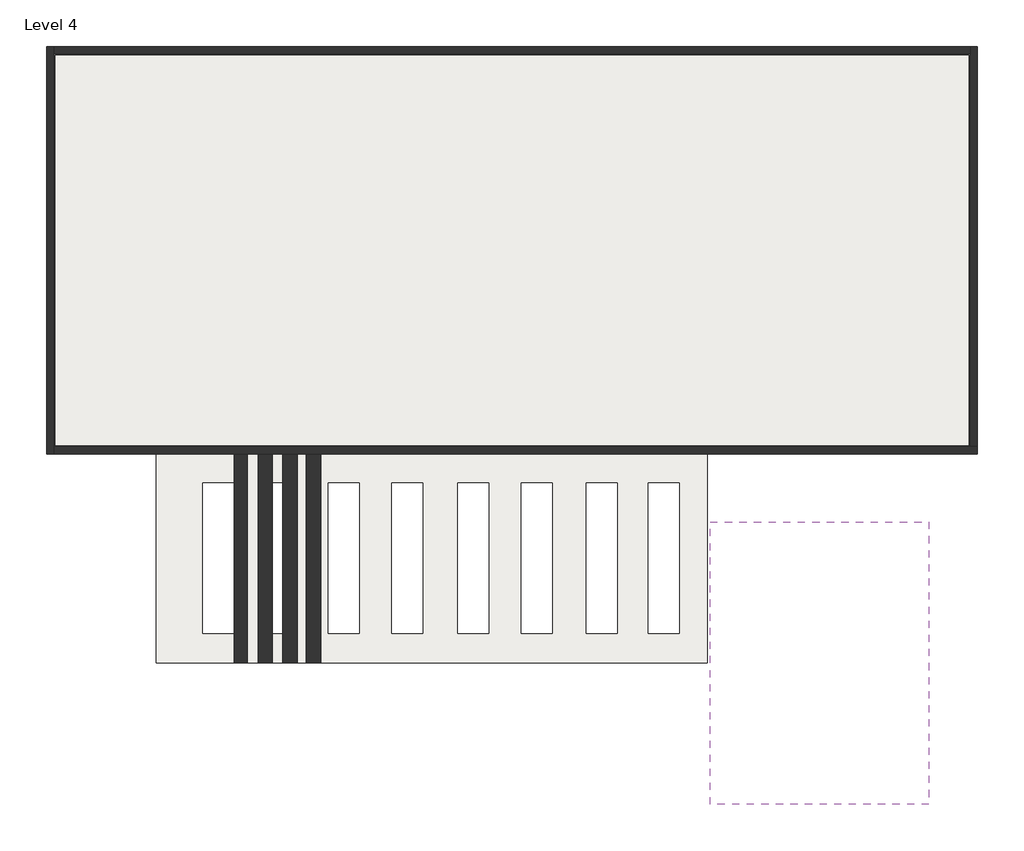
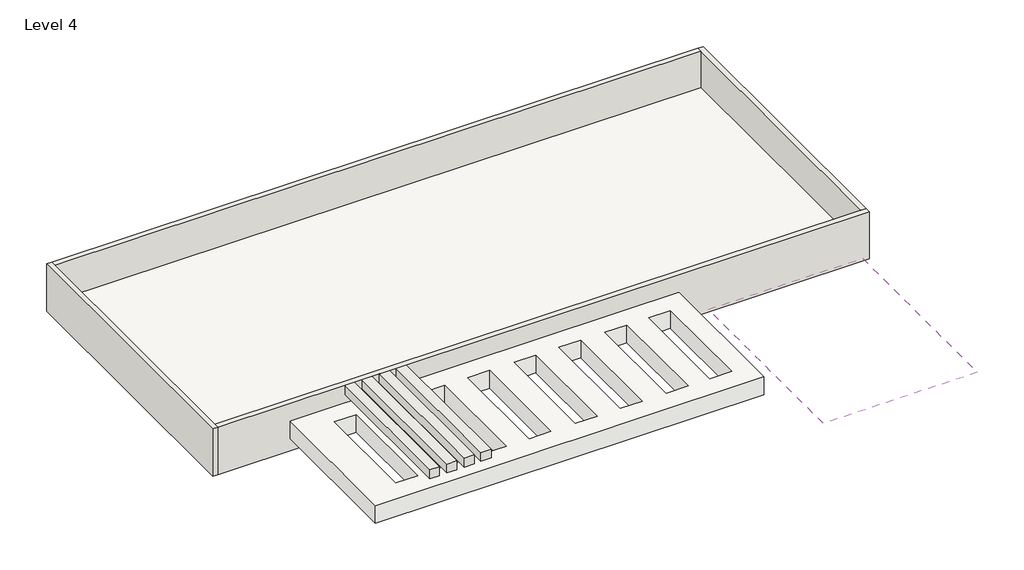
# One storey, incomplete: 5 walls, 3 roofs.
"""IFC4 building model written with IfcOpenShell, lengths in millimetres."""

from ifc_helpers import new_model, si_unit, frame, origin, place, context, project, spatial, polyline, outline, extrude, faceted_brep, transform, mapped, element, save
from components import walls_7_walls_7_6bd86e60

model = new_model("IFC4")

# Units and contexts
model_context = context("Model", 3, world=origin())
ifc_project = project(units=[si_unit("LENGTHUNIT", "METRE", prefix="MILLI")], contexts=[model_context])

# Site, building, storey
site = spatial("IfcSite", under=ifc_project)
building = spatial("IfcBuilding", under=site)
storey = spatial("IfcBuildingStorey", under=building, Name="Level 4", Elevation=10972.8)

# Roofs
placement = place(None, origin())
element("IfcRoof", 1, ObjectType="Generic - 12\"", at=placement, inside=storey, context=model_context, shape_type="SweptSolid", body=[
    extrude(outline(polyline([(-11592.9602581, 8068.7114178), (4110.5897419, 8068.7114178), (4110.5897419, 1363.1114178), (-11592.9602581, 1363.1114178), (-11592.9602581, 8068.7114178)])), frame((0.0, 0.0, 10972.8), z_axis=(0.0, 0.0, 1.0), x_axis=(1.0, 0.0, 0.0)), (0.0, 0.0, 1.0), 304.8),
])
element("IfcRoof", 2, ObjectType="Generic - 12\"", at=placement, inside=storey, context=model_context, shape_type="SweptSolid", body=[
    extrude(outline(polyline([(-337.4620963, 42.3114178), (3421.7379037, 42.3114178), (3421.7379037, -4809.0885822), (-337.4620963, -4809.0885822), (-337.4620963, 42.3114178)])), frame((0.0, 0.0, 11988.8), z_axis=(0.0, 0.0, 1.0), x_axis=(1.0, 0.0, 0.0)), (0.0, 0.0, 1.0), 304.8),
])
element("IfcRoof", 3, ObjectType="Generic - 18\"", at=placement, inside=storey, context=model_context, shape_type="SweptSolid", body=[
    extrude(outline(polyline([(-9855.5936547, 1337.7114178), (-388.2620963, 1337.7114178), (-388.2620963, -2383.3885822), (-9855.5936547, -2383.3885822), (-9855.5936547, 1337.7114178)]), holes=[polyline([(-8530.7557758, -1873.0263421), (-8530.7557758, 717.7736579), (-9064.1557758, 717.7736579), (-9064.1557758, -1873.0263421), (-8530.7557758, -1873.0263421)]), polyline([(-7438.5557758, -1873.0263421), (-7438.5557758, 717.7736579), (-7971.9557758, 717.7736579), (-7971.9557758, -1873.0263421), (-7438.5557758, -1873.0263421)]), polyline([(-6371.7557758, -1873.0263421), (-6371.7557758, 717.7736579), (-6905.1557758, 717.7736579), (-6905.1557758, -1873.0263421), (-6371.7557758, -1873.0263421)]), polyline([(-5279.5557758, -1873.0263421), (-5279.5557758, 717.7736579), (-5812.9557758, 717.7736579), (-5812.9557758, -1873.0263421), (-5279.5557758, -1873.0263421)]), polyline([(-4147.4620963, -1873.0263421), (-4147.4620963, 717.7736579), (-4680.8620963, 717.7736579), (-4680.8620963, -1873.0263421), (-4147.4620963, -1873.0263421)]), polyline([(-3055.2620963, -1873.0263421), (-3055.2620963, 717.7736579), (-3588.6620963, 717.7736579), (-3588.6620963, -1873.0263421), (-3055.2620963, -1873.0263421)]), polyline([(-1937.6620963, -1873.0263421), (-1937.6620963, 717.7736579), (-2471.0620963, 717.7736579), (-2471.0620963, -1873.0263421), (-1937.6620963, -1873.0263421)]), polyline([(-870.8620963, -1873.0263421), (-870.8620963, 717.7736579), (-1404.2620963, 717.7736579), (-1404.2620963, -1873.0263421), (-870.8620963, -1873.0263421)])]), frame((0.0, 0.0, 11277.6), z_axis=(0.0, 0.0, 1.0), x_axis=(1.0, 0.0, 0.0)), (0.0, 0.0, 1.0), 457.2),
])

# Walls
element("IfcWall", 4, ObjectType="Generic - 5\"", at=placement, inside=storey, context=model_context, shape_type="Brep", body=[
    faceted_brep([(-11745.3602581, 8221.1114178, 10972.8), (-11745.3602581, 1210.7114178, 10972.8), (-11745.3602581, 1210.7114178, 12192.0), (-11745.3602581, 8221.1114178, 12192.0), (-11618.3602581, 8221.1114178, 10972.8), (-11618.3602581, 8221.1114178, 12192.0), (-11618.3602581, 8094.1114178, 12192.0), (-11618.3602581, 1337.7114178, 12192.0), (-11618.3602581, 1210.7114178, 12192.0), (-11618.3602581, 1210.7114178, 10972.8), (-11618.3602581, 1337.7114178, 10972.8), (-11618.3602581, 8094.1114178, 10972.8)], [[[0, 1, 2, 3]], [[4, 5, 6, 7, 8, 9, 10, 11]], [[1, 0, 4, 11, 10, 9]], [[3, 2, 8, 7, 6, 5]], [[2, 1, 9, 8]], [[0, 3, 5, 4]]]),
])
element("IfcWall", 5, ObjectType="Generic - 5\"", at=placement, inside=storey, context=model_context, shape_type="Brep", body=[
    faceted_brep([(-11618.3602581, 1210.7114178, 10972.8), (4256.6397419, 1210.7114178, 10972.8), (4256.6397419, 1210.7114178, 12192.0), (-11618.3602581, 1210.7114178, 12192.0), (-11618.3602581, 1337.7114178, 10972.8), (-11618.3602581, 1337.7114178, 12192.0), (4129.6397419, 1337.7114178, 12192.0), (4256.6397419, 1337.7114178, 12192.0), (4256.6397419, 1337.7114178, 10972.8), (4129.6397419, 1337.7114178, 10972.8)], [[[0, 1, 2, 3]], [[4, 5, 6, 7, 8, 9]], [[1, 0, 4, 9, 8]], [[3, 2, 7, 6, 5]], [[0, 3, 5, 4]], [[2, 1, 8, 7]]]),
])
element("IfcWall", 6, ObjectType="Generic - 5\"", at=placement, inside=storey, context=model_context, shape_type="Brep", body=[
    faceted_brep([(4256.6397419, 1337.7114178, 10972.8), (4256.6397419, 8221.1114178, 10972.8), (4256.6397419, 8221.1114178, 12192.0), (4256.6397419, 1337.7114178, 12192.0), (4129.6397419, 1337.7114178, 10972.8), (4129.6397419, 1337.7114178, 12192.0), (4129.6397419, 8094.1114178, 12192.0), (4129.6397419, 8221.1114178, 12192.0), (4129.6397419, 8221.1114178, 10972.8), (4129.6397419, 8094.1114178, 10972.8)], [[[0, 1, 2, 3]], [[4, 5, 6, 7, 8, 9]], [[1, 0, 4, 9, 8]], [[3, 2, 7, 6, 5]], [[0, 3, 5, 4]], [[2, 1, 8, 7]]]),
])
element("IfcWall", 7, ObjectType="Generic - 5\"", at=placement, inside=storey, context=model_context, shape_type="SweptSolid", body=[
    extrude(outline(polyline([(-11618.3602581, 8221.1114178), (4129.6397419, 8221.1114178), (4129.6397419, 8094.1114178), (-11618.3602581, 8094.1114178), (-11618.3602581, 8221.1114178)])), frame((0.0, 0.0, 10972.8), z_axis=(0.0, 0.0, 1.0), x_axis=(1.0, 0.0, 0.0)), (0.0, 0.0, 1.0), 1219.2),
])
walls_7_walls_7_shape = walls_7_walls_7_6bd86e60(model_context)
element("IfcWall", 8, ObjectType="Walls 7 : Walls 7", at=placement, inside=storey, context=model_context, shape_type="MappedRepresentation", body=[
    mapped(walls_7_walls_7_shape, transform((0.0, 0.0, 0.0), x_axis=(1.0, 0.0, 0.0), y_axis=(0.0, 1.0, 0.0), z_axis=(0.0, 0.0, 1.0))),
])

save(model, "model.ifc")

# Revit data of these elements
# Type "Generic - 12\""
#   Assembly Code = "B1020"
#   Layers, outside or top first: 1' - 0" no material (function 1)
# Type "Generic - 18\""
#   Assembly Code = "B1020"
#   Layers, outside or top first: 1' - 6" no material (function 1)
# Type "Generic - 5\""
#   Assembly Code = "B2010"
#   Layers, outside or top first: 0' - 5" no material (function 1)
# Element 1 (IfcRoof, "Generic - 12\"")
#   built-in parameter 1001705 = 37 (stored number, unit not read)
#   built-in parameter 1001710 = 33615
#   Phase Created = New Construction
#   Materials on its faces: "Default Roof"
# Element 2 (IfcRoof, "Generic - 12\"")
#   built-in parameter 1001705 = 40.3333 (stored number, unit not read)
#   built-in parameter 1001701 = 3.33333 (stored number, unit not read)
#   built-in parameter 1001710 = 33615
#   Phase Created = New Construction
#   Materials on its faces: "Default Roof"
# Element 3 (IfcRoof, "Generic - 18\"")
#   built-in parameter 1001705 = 38.5 (stored number, unit not read)
#   built-in parameter 1001701 = 1 (stored number, unit not read)
#   built-in parameter 1001710 = 33615
#   Phase Created = New Construction
#   Materials on its faces: "Default Roof"
# Elements 4, 5, 6, 7 (IfcWall, "Generic - 5\"")
#   Top Offset = -8' - 0"
#   Base Offset = 0' - 0"
#   wall height = 4' - 0"
#   Phase Created = New Construction
#   Base Constraint = Level 4
#   Top Constraint = Level 5
#   Materials on its faces: "Default Wall"
# Element 8 (IfcWall, "Walls 7 : Walls 7")
#   Phase Created = New Construction
#   Materials on its faces: "Default Wall"
# Materials
#   "Default Roof": colour RGB 88 101 114, transparency 0
#   "Default Wall": colour RGB 128 128 128, transparency 0
